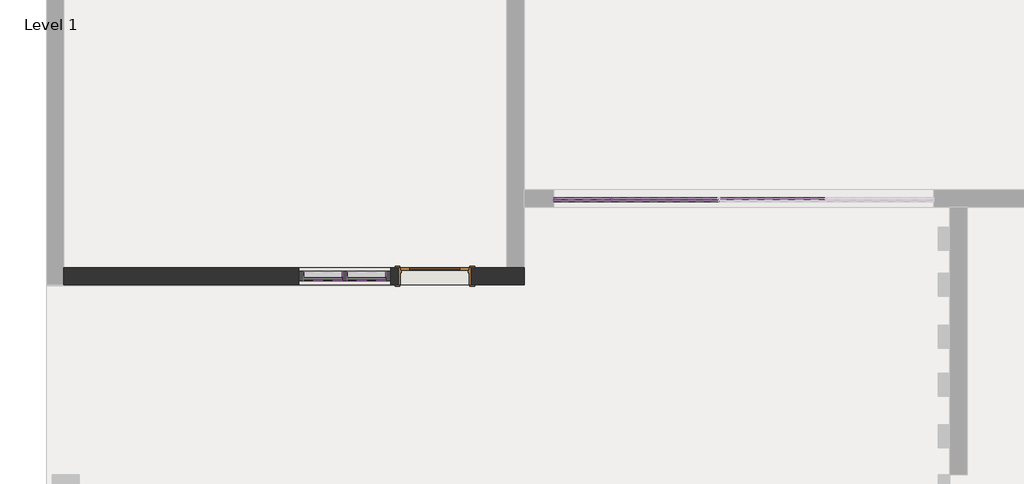
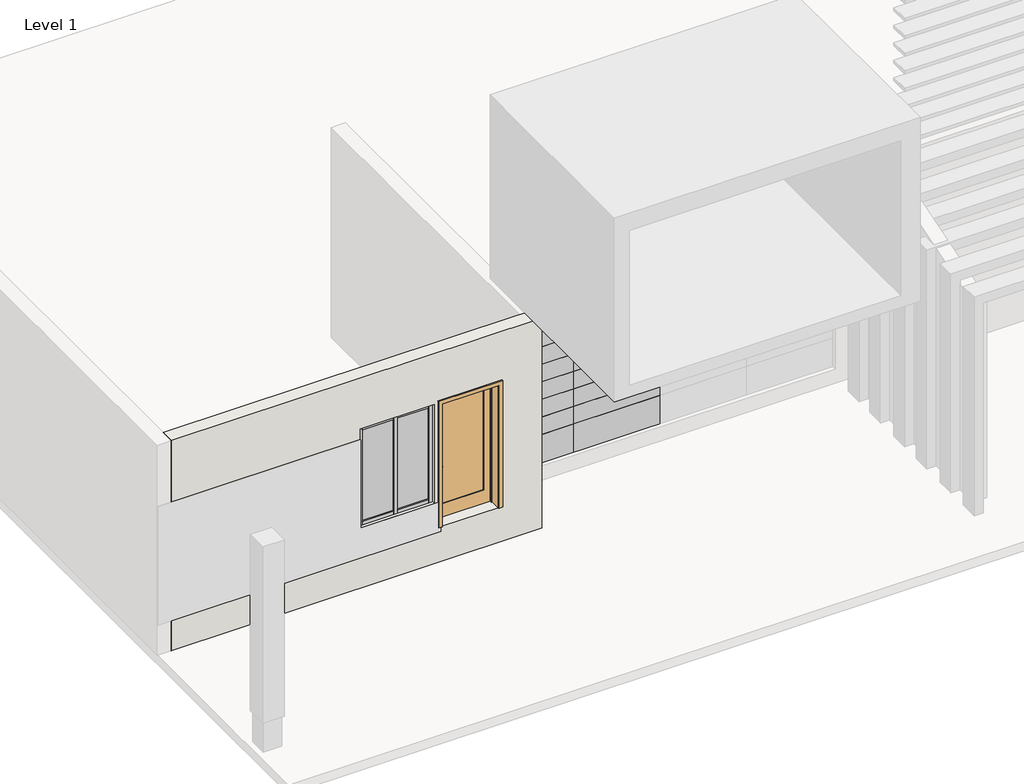
# One storey, part 1 of 2: 50 members, 18 plates, 1 door, 1 wall.
"""IFC4 building model written with IfcOpenShell, lengths in millimetres."""

from ifc_helpers import new_model, si_unit, origin, place, context, project, spatial, faceted_brep, transform, mapped, element, save
from components import door_interior_single_1_panel_wood_3_x_7_3b97b8e7, member_f362a377, member_550490f7, member_dc2600c8, member_5ac041f4, member_20a2445f, member_63f4cac5, member_d020295e, member_84e80635, member_b7a731ef, member_839e3c67, member_0b7646a3, member_58564e40, member_14ac651b, system_panel_glazed_f636780f, system_panel_glazed_497abead, system_panel_glazed_074527c7, system_panel_glazed_4c8acbbb, system_panel_glazed_d4e05dc3, system_panel_glazed_d663d970, system_panel_glazed_cac74210

model = new_model("IFC4")

# Units and contexts
model_context = context("Model", 3, world=origin())
ifc_project = project(units=[si_unit("LENGTHUNIT", "METRE", prefix="MILLI")], contexts=[model_context])

# Site, building, storey
site = spatial("IfcSite", under=ifc_project)
building = spatial("IfcBuilding", under=site)
storey = spatial("IfcBuildingStorey", under=building, Name="Level 1", Elevation=0.0)

# Door
placement = place(None, origin())
door_interior_single_1_panel_wood_3_x_7_shape = door_interior_single_1_panel_wood_3_x_7_3b97b8e7(model_context)
element("IfcDoor", 1, ObjectType="Door-Interior-Single-1_Panel-Wood : 3' x 7'", at=placement, inside=storey, context=model_context, shape_type="MappedRepresentation", body=[
    mapped(door_interior_single_1_panel_wood_3_x_7_shape, transform((-8192.4294011, -2264.4361529, 609.6), x_axis=(1.0, 0.0, 0.0), y_axis=(0.0, 1.0, 0.0), z_axis=(0.0, 0.0, 1.0))),
])

# Members
member_shape = member_f362a377(model_context)
element("IfcMember", 2, ObjectType="Rectangular Mullion : 1\" Square", at=placement, inside=storey, context=model_context, shape_type="MappedRepresentation", body=[
    mapped(member_shape, transform((-6592.2294011, -1238.9111529, 2823.4928635), x_axis=(0.0, 0.0, 1.0), y_axis=(0.0, 1.0, 0.0), z_axis=(-1.0, 0.0, 0.0))),
])
member_2_shape = member_550490f7(model_context)
element("IfcMember", 3, ObjectType="Rectangular Mullion : 1\" Square", at=placement, inside=storey, context=model_context, shape_type="MappedRepresentation", body=[
    mapped(member_2_shape, transform((-6592.2294011, -1238.9111529, 2572.3741932), x_axis=(0.0, 0.0, 1.0), y_axis=(0.0, 1.0, 0.0), z_axis=(-1.0, 0.0, 0.0))),
])
element("IfcMember", 4, ObjectType="Rectangular Mullion : 1\" Square", at=placement, inside=storey, context=model_context, shape_type="MappedRepresentation", body=[
    mapped(member_2_shape, transform((-6592.2294011, -1238.9111529, 2267.5741932), x_axis=(0.0, 0.0, 1.0), y_axis=(0.0, 1.0, 0.0), z_axis=(-1.0, 0.0, 0.0))),
])
element("IfcMember", 5, ObjectType="Rectangular Mullion : 1\" Square", at=placement, inside=storey, context=model_context, shape_type="MappedRepresentation", body=[
    mapped(member_2_shape, transform((-6592.2294011, -1238.9111529, 1962.7741932), x_axis=(0.0, 0.0, 1.0), y_axis=(0.0, 1.0, 0.0), z_axis=(-1.0, 0.0, 0.0))),
])
element("IfcMember", 6, ObjectType="Rectangular Mullion : 1\" Square", at=placement, inside=storey, context=model_context, shape_type="MappedRepresentation", body=[
    mapped(member_2_shape, transform((-6592.2294011, -1238.9111529, 1353.1741932), x_axis=(0.0, 0.0, 1.0), y_axis=(0.0, 1.0, 0.0), z_axis=(-1.0, 0.0, 0.0))),
])
element("IfcMember", 7, ObjectType="Rectangular Mullion : 1\" Square", at=placement, inside=storey, context=model_context, shape_type="MappedRepresentation", body=[
    mapped(member_2_shape, transform((-6592.2294011, -1238.9111529, 1657.9741932), x_axis=(0.0, 0.0, 1.0), y_axis=(0.0, 1.0, 0.0), z_axis=(-1.0, 0.0, 0.0))),
])
element("IfcMember", 8, ObjectType="Rectangular Mullion : 1\" Square", at=placement, inside=storey, context=model_context, shape_type="MappedRepresentation", body=[
    mapped(member_2_shape, transform((-6592.2294011, -1238.9111529, 1048.3741932), x_axis=(0.0, 0.0, 1.0), y_axis=(0.0, 1.0, 0.0), z_axis=(-1.0, 0.0, 0.0))),
])
element("IfcMember", 9, ObjectType="Rectangular Mullion : 1\" Square", at=placement, inside=storey, context=model_context, shape_type="MappedRepresentation", body=[
    mapped(member_2_shape, transform((-6592.2294011, -1238.9111529, 743.5741932), x_axis=(0.0, 0.0, 1.0), y_axis=(0.0, 1.0, 0.0), z_axis=(-1.0, 0.0, 0.0))),
])
member_3_shape = member_dc2600c8(model_context)
element("IfcMember", 10, ObjectType="Rectangular Mullion : 1\" Square", at=placement, inside=storey, context=model_context, shape_type="MappedRepresentation", body=[
    mapped(member_3_shape, transform((-5842.9294011, -1238.9111529, 2572.3741932), x_axis=(0.0, 0.0, 1.0), y_axis=(0.0, 1.0, 0.0), z_axis=(-1.0, 0.0, 0.0))),
])
element("IfcMember", 11, ObjectType="Rectangular Mullion : 1\" Square", at=placement, inside=storey, context=model_context, shape_type="MappedRepresentation", body=[
    mapped(member_3_shape, transform((-4420.5294011, -1238.9111529, 2572.3741932), x_axis=(0.0, 0.0, 1.0), y_axis=(0.0, 1.0, 0.0), z_axis=(-1.0, 0.0, 0.0))),
])
element("IfcMember", 12, ObjectType="Rectangular Mullion : 1\" Square", at=placement, inside=storey, context=model_context, shape_type="MappedRepresentation", body=[
    mapped(member_3_shape, transform((-5842.9294011, -1238.9111529, 2267.5741932), x_axis=(0.0, 0.0, 1.0), y_axis=(0.0, 1.0, 0.0), z_axis=(-1.0, 0.0, 0.0))),
])
element("IfcMember", 13, ObjectType="Rectangular Mullion : 1\" Square", at=placement, inside=storey, context=model_context, shape_type="MappedRepresentation", body=[
    mapped(member_3_shape, transform((-4420.5294011, -1238.9111529, 2267.5741932), x_axis=(0.0, 0.0, 1.0), y_axis=(0.0, 1.0, 0.0), z_axis=(-1.0, 0.0, 0.0))),
])
element("IfcMember", 14, ObjectType="Rectangular Mullion : 1\" Square", at=placement, inside=storey, context=model_context, shape_type="MappedRepresentation", body=[
    mapped(member_3_shape, transform((-5842.9294011, -1238.9111529, 1962.7741932), x_axis=(0.0, 0.0, 1.0), y_axis=(0.0, 1.0, 0.0), z_axis=(-1.0, 0.0, 0.0))),
])
element("IfcMember", 15, ObjectType="Rectangular Mullion : 1\" Square", at=placement, inside=storey, context=model_context, shape_type="MappedRepresentation", body=[
    mapped(member_3_shape, transform((-4420.5294011, -1238.9111529, 1962.7741932), x_axis=(0.0, 0.0, 1.0), y_axis=(0.0, 1.0, 0.0), z_axis=(-1.0, 0.0, 0.0))),
])
element("IfcMember", 16, ObjectType="Rectangular Mullion : 1\" Square", at=placement, inside=storey, context=model_context, shape_type="MappedRepresentation", body=[
    mapped(member_3_shape, transform((-5842.9294011, -1238.9111529, 1353.1741932), x_axis=(0.0, 0.0, 1.0), y_axis=(0.0, 1.0, 0.0), z_axis=(-1.0, 0.0, 0.0))),
])
element("IfcMember", 17, ObjectType="Rectangular Mullion : 1\" Square", at=placement, inside=storey, context=model_context, shape_type="MappedRepresentation", body=[
    mapped(member_3_shape, transform((-4420.5294011, -1238.9111529, 1353.1741932), x_axis=(0.0, 0.0, 1.0), y_axis=(0.0, 1.0, 0.0), z_axis=(-1.0, 0.0, 0.0))),
])
element("IfcMember", 18, ObjectType="Rectangular Mullion : 1\" Square", at=placement, inside=storey, context=model_context, shape_type="MappedRepresentation", body=[
    mapped(member_3_shape, transform((-5842.9294011, -1238.9111529, 1657.9741932), x_axis=(0.0, 0.0, 1.0), y_axis=(0.0, 1.0, 0.0), z_axis=(-1.0, 0.0, 0.0))),
])
element("IfcMember", 19, ObjectType="Rectangular Mullion : 1\" Square", at=placement, inside=storey, context=model_context, shape_type="MappedRepresentation", body=[
    mapped(member_3_shape, transform((-4420.5294011, -1238.9111529, 1657.9741932), x_axis=(0.0, 0.0, 1.0), y_axis=(0.0, 1.0, 0.0), z_axis=(-1.0, 0.0, 0.0))),
])
element("IfcMember", 20, ObjectType="Rectangular Mullion : 1\" Square", at=placement, inside=storey, context=model_context, shape_type="MappedRepresentation", body=[
    mapped(member_3_shape, transform((-5842.9294011, -1238.9111529, 1048.3741932), x_axis=(0.0, 0.0, 1.0), y_axis=(0.0, 1.0, 0.0), z_axis=(-1.0, 0.0, 0.0))),
])
element("IfcMember", 21, ObjectType="Rectangular Mullion : 1\" Square", at=placement, inside=storey, context=model_context, shape_type="MappedRepresentation", body=[
    mapped(member_3_shape, transform((-4420.5294011, -1238.9111529, 1048.3741932), x_axis=(0.0, 0.0, 1.0), y_axis=(0.0, 1.0, 0.0), z_axis=(-1.0, 0.0, 0.0))),
])
element("IfcMember", 22, ObjectType="Rectangular Mullion : 1\" Square", at=placement, inside=storey, context=model_context, shape_type="MappedRepresentation", body=[
    mapped(member_3_shape, transform((-5842.9294011, -1238.9111529, 743.5741932), x_axis=(0.0, 0.0, 1.0), y_axis=(0.0, 1.0, 0.0), z_axis=(-1.0, 0.0, 0.0))),
])
element("IfcMember", 23, ObjectType="Rectangular Mullion : 1\" Square", at=placement, inside=storey, context=model_context, shape_type="MappedRepresentation", body=[
    mapped(member_3_shape, transform((-4420.5294011, -1238.9111529, 743.5741932), x_axis=(0.0, 0.0, 1.0), y_axis=(0.0, 1.0, 0.0), z_axis=(-1.0, 0.0, 0.0))),
])
member_4_shape = member_5ac041f4(model_context)
element("IfcMember", 24, ObjectType="Rectangular Mullion : 1\" Square", at=placement, inside=storey, context=model_context, shape_type="MappedRepresentation", body=[
    mapped(member_4_shape, transform((-5855.6294011, -1238.9111529, 247.9343309), x_axis=(-1.0, 0.0, 0.0), y_axis=(0.0, 1.0, 0.0), z_axis=(0.0, 0.0, -1.0))),
])
element("IfcMember", 25, ObjectType="Rectangular Mullion : 1\" Square", at=placement, inside=storey, context=model_context, shape_type="MappedRepresentation", body=[
    mapped(member_4_shape, transform((-4433.2294011, -1238.9111529, 247.9343309), x_axis=(-1.0, 0.0, 0.0), y_axis=(0.0, 1.0, 0.0), z_axis=(0.0, 0.0, -1.0))),
])
element("IfcMember", 26, ObjectType="Rectangular Mullion : 1\" Square", at=placement, inside=storey, context=model_context, shape_type="MappedRepresentation", body=[
    mapped(member_shape, transform((-5868.3294011, -1238.9111529, 247.9343309), x_axis=(0.0, 0.0, -1.0), y_axis=(0.0, 1.0, 0.0), z_axis=(1.0, 0.0, 0.0))),
])
member_5_shape = member_20a2445f(model_context)
element("IfcMember", 27, ObjectType="Rectangular Mullion : 1\" Square", at=placement, inside=storey, context=model_context, shape_type="MappedRepresentation", body=[
    mapped(member_5_shape, transform((-4445.9294011, -1238.9111529, 247.9343309), x_axis=(0.0, 0.0, -1.0), y_axis=(0.0, 1.0, 0.0), z_axis=(1.0, 0.0, 0.0))),
])
element("IfcMember", 28, ObjectType="Rectangular Mullion : 1\" Square", at=placement, inside=storey, context=model_context, shape_type="MappedRepresentation", body=[
    mapped(member_5_shape, transform((-5842.9294011, -1238.9111529, 2823.4928635), x_axis=(0.0, 0.0, 1.0), y_axis=(0.0, 1.0, 0.0), z_axis=(-1.0, 0.0, 0.0))),
])
element("IfcMember", 29, ObjectType="Rectangular Mullion : 1\" Square", at=placement, inside=storey, context=model_context, shape_type="MappedRepresentation", body=[
    mapped(member_5_shape, transform((-4420.5294011, -1238.9111529, 2823.4928635), x_axis=(0.0, 0.0, 1.0), y_axis=(0.0, 1.0, 0.0), z_axis=(-1.0, 0.0, 0.0))),
])
member_6_shape = member_63f4cac5(model_context)
element("IfcMember", 30, ObjectType="Rectangular Mullion : 1\" Square", at=placement, inside=storey, context=model_context, shape_type="MappedRepresentation", body=[
    mapped(member_6_shape, transform((-5855.6294011, -1238.9111529, 2572.3741932), x_axis=(-1.0, 0.0, 0.0), y_axis=(0.0, 1.0, 0.0), z_axis=(0.0, 0.0, -1.0))),
])
member_7_shape = member_d020295e(model_context)
element("IfcMember", 31, ObjectType="Rectangular Mullion : 1\" Square", at=placement, inside=storey, context=model_context, shape_type="MappedRepresentation", body=[
    mapped(member_7_shape, transform((-5855.6294011, -1238.9111529, 2267.5741932), x_axis=(-1.0, 0.0, 0.0), y_axis=(0.0, 1.0, 0.0), z_axis=(0.0, 0.0, -1.0))),
])
element("IfcMember", 32, ObjectType="Rectangular Mullion : 1\" Square", at=placement, inside=storey, context=model_context, shape_type="MappedRepresentation", body=[
    mapped(member_7_shape, transform((-5855.6294011, -1238.9111529, 1962.7741932), x_axis=(-1.0, 0.0, 0.0), y_axis=(0.0, 1.0, 0.0), z_axis=(0.0, 0.0, -1.0))),
])
element("IfcMember", 33, ObjectType="Rectangular Mullion : 1\" Square", at=placement, inside=storey, context=model_context, shape_type="MappedRepresentation", body=[
    mapped(member_7_shape, transform((-5855.6294011, -1238.9111529, 1353.1741932), x_axis=(-1.0, 0.0, 0.0), y_axis=(0.0, 1.0, 0.0), z_axis=(0.0, 0.0, -1.0))),
])
element("IfcMember", 34, ObjectType="Rectangular Mullion : 1\" Square", at=placement, inside=storey, context=model_context, shape_type="MappedRepresentation", body=[
    mapped(member_7_shape, transform((-5855.6294011, -1238.9111529, 1657.9741932), x_axis=(-1.0, 0.0, 0.0), y_axis=(0.0, 1.0, 0.0), z_axis=(0.0, 0.0, -1.0))),
])
element("IfcMember", 35, ObjectType="Rectangular Mullion : 1\" Square", at=placement, inside=storey, context=model_context, shape_type="MappedRepresentation", body=[
    mapped(member_7_shape, transform((-5855.6294011, -1238.9111529, 1048.3741932), x_axis=(-1.0, 0.0, 0.0), y_axis=(0.0, 1.0, 0.0), z_axis=(0.0, 0.0, -1.0))),
])
element("IfcMember", 36, ObjectType="Rectangular Mullion : 1\" Square", at=placement, inside=storey, context=model_context, shape_type="MappedRepresentation", body=[
    mapped(member_7_shape, transform((-5855.6294011, -1238.9111529, 743.5741932), x_axis=(-1.0, 0.0, 0.0), y_axis=(0.0, 1.0, 0.0), z_axis=(0.0, 0.0, -1.0))),
])
member_8_shape = member_84e80635(model_context)
element("IfcMember", 37, ObjectType="Rectangular Mullion : 1\" Square", at=placement, inside=storey, context=model_context, shape_type="MappedRepresentation", body=[
    mapped(member_8_shape, transform((-6617.6294011, -1238.9111529, 247.9343309), x_axis=(-1.0, 0.0, 0.0), y_axis=(0.0, 1.0, 0.0), z_axis=(0.0, 0.0, -1.0))),
])
member_9_shape = member_b7a731ef(model_context)
element("IfcMember", 38, ObjectType="Rectangular Mullion : 1\" Square", at=placement, inside=storey, context=model_context, shape_type="MappedRepresentation", body=[
    mapped(member_9_shape, transform((-6617.6294011, -1238.9111529, 2572.3741932), x_axis=(-1.0, 0.0, 0.0), y_axis=(0.0, 1.0, 0.0), z_axis=(0.0, 0.0, -1.0))),
])
member_10_shape = member_839e3c67(model_context)
element("IfcMember", 39, ObjectType="Rectangular Mullion : 1\" Square", at=placement, inside=storey, context=model_context, shape_type="MappedRepresentation", body=[
    mapped(member_10_shape, transform((-6617.6294011, -1238.9111529, 2267.5741932), x_axis=(-1.0, 0.0, 0.0), y_axis=(0.0, 1.0, 0.0), z_axis=(0.0, 0.0, -1.0))),
])
element("IfcMember", 40, ObjectType="Rectangular Mullion : 1\" Square", at=placement, inside=storey, context=model_context, shape_type="MappedRepresentation", body=[
    mapped(member_10_shape, transform((-6617.6294011, -1238.9111529, 1962.7741932), x_axis=(-1.0, 0.0, 0.0), y_axis=(0.0, 1.0, 0.0), z_axis=(0.0, 0.0, -1.0))),
])
element("IfcMember", 41, ObjectType="Rectangular Mullion : 1\" Square", at=placement, inside=storey, context=model_context, shape_type="MappedRepresentation", body=[
    mapped(member_10_shape, transform((-6617.6294011, -1238.9111529, 1353.1741932), x_axis=(-1.0, 0.0, 0.0), y_axis=(0.0, 1.0, 0.0), z_axis=(0.0, 0.0, -1.0))),
])
element("IfcMember", 42, ObjectType="Rectangular Mullion : 1\" Square", at=placement, inside=storey, context=model_context, shape_type="MappedRepresentation", body=[
    mapped(member_10_shape, transform((-6617.6294011, -1238.9111529, 1657.9741932), x_axis=(-1.0, 0.0, 0.0), y_axis=(0.0, 1.0, 0.0), z_axis=(0.0, 0.0, -1.0))),
])
element("IfcMember", 43, ObjectType="Rectangular Mullion : 1\" Square", at=placement, inside=storey, context=model_context, shape_type="MappedRepresentation", body=[
    mapped(member_10_shape, transform((-6617.6294011, -1238.9111529, 1048.3741932), x_axis=(-1.0, 0.0, 0.0), y_axis=(0.0, 1.0, 0.0), z_axis=(0.0, 0.0, -1.0))),
])
element("IfcMember", 44, ObjectType="Rectangular Mullion : 1\" Square", at=placement, inside=storey, context=model_context, shape_type="MappedRepresentation", body=[
    mapped(member_10_shape, transform((-6617.6294011, -1238.9111529, 743.5741932), x_axis=(-1.0, 0.0, 0.0), y_axis=(0.0, 1.0, 0.0), z_axis=(0.0, 0.0, -1.0))),
])
member_11_shape = member_0b7646a3(model_context)
element("IfcMember", 45, ObjectType="Rectangular Mullion : 2.5\" x 5\" rectangular 2", at=placement, inside=storey, context=model_context, shape_type="MappedRepresentation", body=[
    mapped(member_11_shape, transform((-9932.3294011, -2267.6111529, 2768.6), x_axis=(0.0, 0.0, 1.0), y_axis=(0.0, 1.0, 0.0), z_axis=(-1.0, 0.0, 0.0))),
])
element("IfcMember", 46, ObjectType="Rectangular Mullion : 2.5\" x 5\" rectangular 2", at=placement, inside=storey, context=model_context, shape_type="MappedRepresentation", body=[
    mapped(member_11_shape, transform((-9354.4794011, -2267.6111529, 2768.6), x_axis=(0.0, 0.0, 1.0), y_axis=(0.0, 1.0, 0.0), z_axis=(-1.0, 0.0, 0.0))),
])
element("IfcMember", 47, ObjectType="Rectangular Mullion : 2.5\" x 5\" rectangular 2", at=placement, inside=storey, context=model_context, shape_type="MappedRepresentation", body=[
    mapped(member_11_shape, transform((-8840.1294011, -2267.6111529, 1047.6775384), x_axis=(0.0, 0.0, -1.0), y_axis=(0.0, 1.0, 0.0), z_axis=(1.0, 0.0, 0.0))),
])
element("IfcMember", 48, ObjectType="Rectangular Mullion : 2.5\" x 5\" rectangular 2", at=placement, inside=storey, context=model_context, shape_type="MappedRepresentation", body=[
    mapped(member_11_shape, transform((-9417.9794011, -2267.6111529, 1047.6775384), x_axis=(0.0, 0.0, -1.0), y_axis=(0.0, 1.0, 0.0), z_axis=(1.0, 0.0, 0.0))),
])
member_12_shape = member_58564e40(model_context)
element("IfcMember", 49, ObjectType="Rectangular Mullion : 2.5\" x 5\" rectangular 2", at=placement, inside=storey, context=model_context, shape_type="MappedRepresentation", body=[
    mapped(member_12_shape, transform((-9386.2294011, -2267.6111529, 1047.6775384), x_axis=(-1.0, 0.0, 0.0), y_axis=(0.0, 1.0, 0.0), z_axis=(0.0, 0.0, -1.0))),
])
member_13_shape = member_14ac651b(model_context)
element("IfcMember", 50, ObjectType="Rectangular Mullion : 2.5\" x 5\" rectangular 2", at=placement, inside=storey, context=model_context, shape_type="MappedRepresentation", body=[
    mapped(member_13_shape, transform((-8776.6294011, -2267.6111529, 2768.6), x_axis=(1.0, 0.0, 0.0), y_axis=(0.0, 1.0, 0.0), z_axis=(0.0, 0.0, 1.0))),
])
element("IfcMember", 51, ObjectType="Rectangular Mullion : 2.5\" x 5\" rectangular 2", at=placement, inside=storey, context=model_context, shape_type="MappedRepresentation", body=[
    mapped(member_13_shape, transform((-9995.8294011, -2267.6111529, 1047.6775384), x_axis=(-1.0, 0.0, 0.0), y_axis=(0.0, 1.0, 0.0), z_axis=(0.0, 0.0, -1.0))),
])

# Plates
system_panel_glazed_shape = system_panel_glazed_f636780f(model_context)
element("IfcPlate", 52, ObjectType="System Panel : Glazed", at=placement, inside=storey, context=model_context, shape_type="MappedRepresentation", body=[
    mapped(system_panel_glazed_shape, transform((-9097.3044011, -2267.6111529, 1111.1775384), x_axis=(-1.0, 0.0, 0.0), y_axis=(0.0, -1.0, 0.0), z_axis=(0.0, 0.0, 1.0))),
])
element("IfcPlate", 53, ObjectType="System Panel : Glazed", at=placement, inside=storey, context=model_context, shape_type="MappedRepresentation", body=[
    mapped(system_panel_glazed_shape, transform((-9675.1544011, -2267.6111529, 1111.1775384), x_axis=(-1.0, 0.0, 0.0), y_axis=(0.0, -1.0, 0.0), z_axis=(0.0, 0.0, 1.0))),
])
system_panel_glazed_2_shape = system_panel_glazed_497abead(model_context)
element("IfcPlate", 54, ObjectType="System Panel : Glazed", at=placement, inside=storey, context=model_context, shape_type="MappedRepresentation", body=[
    mapped(system_panel_glazed_2_shape, transform((-6236.6294011, -1238.9111529, 247.9343309), x_axis=(-1.0, 0.0, 0.0), y_axis=(0.0, -1.0, 0.0), z_axis=(0.0, 0.0, 1.0))),
])
system_panel_glazed_3_shape = system_panel_glazed_074527c7(model_context)
element("IfcPlate", 55, ObjectType="System Panel : Glazed", at=placement, inside=storey, context=model_context, shape_type="MappedRepresentation", body=[
    mapped(system_panel_glazed_3_shape, transform((-6236.6294011, -1238.9111529, 743.5741932), x_axis=(-1.0, 0.0, 0.0), y_axis=(0.0, -1.0, 0.0), z_axis=(0.0, 0.0, 1.0))),
])
element("IfcPlate", 56, ObjectType="System Panel : Glazed", at=placement, inside=storey, context=model_context, shape_type="MappedRepresentation", body=[
    mapped(system_panel_glazed_3_shape, transform((-6236.6294011, -1238.9111529, 1048.3741932), x_axis=(-1.0, 0.0, 0.0), y_axis=(0.0, -1.0, 0.0), z_axis=(0.0, 0.0, 1.0))),
])
element("IfcPlate", 57, ObjectType="System Panel : Glazed", at=placement, inside=storey, context=model_context, shape_type="MappedRepresentation", body=[
    mapped(system_panel_glazed_3_shape, transform((-6236.6294011, -1238.9111529, 1353.1741932), x_axis=(-1.0, 0.0, 0.0), y_axis=(0.0, -1.0, 0.0), z_axis=(0.0, 0.0, 1.0))),
])
element("IfcPlate", 58, ObjectType="System Panel : Glazed", at=placement, inside=storey, context=model_context, shape_type="MappedRepresentation", body=[
    mapped(system_panel_glazed_3_shape, transform((-6236.6294011, -1238.9111529, 1657.9741932), x_axis=(-1.0, 0.0, 0.0), y_axis=(0.0, -1.0, 0.0), z_axis=(0.0, 0.0, 1.0))),
])
element("IfcPlate", 59, ObjectType="System Panel : Glazed", at=placement, inside=storey, context=model_context, shape_type="MappedRepresentation", body=[
    mapped(system_panel_glazed_3_shape, transform((-6236.6294011, -1238.9111529, 1962.7741932), x_axis=(-1.0, 0.0, 0.0), y_axis=(0.0, -1.0, 0.0), z_axis=(0.0, 0.0, 1.0))),
])
element("IfcPlate", 60, ObjectType="System Panel : Glazed", at=placement, inside=storey, context=model_context, shape_type="MappedRepresentation", body=[
    mapped(system_panel_glazed_3_shape, transform((-6236.6294011, -1238.9111529, 2267.5741932), x_axis=(-1.0, 0.0, 0.0), y_axis=(0.0, -1.0, 0.0), z_axis=(0.0, 0.0, 1.0))),
])
system_panel_glazed_4_shape = system_panel_glazed_4c8acbbb(model_context)
element("IfcPlate", 61, ObjectType="System Panel : Glazed", at=placement, inside=storey, context=model_context, shape_type="MappedRepresentation", body=[
    mapped(system_panel_glazed_4_shape, transform((-6236.6294011, -1238.9111529, 2572.3741932), x_axis=(-1.0, 0.0, 0.0), y_axis=(0.0, -1.0, 0.0), z_axis=(0.0, 0.0, 1.0))),
])
system_panel_glazed_5_shape = system_panel_glazed_d4e05dc3(model_context)
element("IfcPlate", 62, ObjectType="System Panel : Glazed", at=placement, inside=storey, context=model_context, shape_type="MappedRepresentation", body=[
    mapped(system_panel_glazed_5_shape, transform((-5144.4294011, -1238.9111529, 247.9343309), x_axis=(-1.0, 0.0, 0.0), y_axis=(0.0, -1.0, 0.0), z_axis=(0.0, 0.0, 1.0))),
])
system_panel_glazed_6_shape = system_panel_glazed_d663d970(model_context)
element("IfcPlate", 63, ObjectType="System Panel : Glazed", at=placement, inside=storey, context=model_context, shape_type="MappedRepresentation", body=[
    mapped(system_panel_glazed_6_shape, transform((-5144.4294011, -1238.9111529, 743.5741932), x_axis=(-1.0, 0.0, 0.0), y_axis=(0.0, -1.0, 0.0), z_axis=(0.0, 0.0, 1.0))),
])
element("IfcPlate", 64, ObjectType="System Panel : Glazed", at=placement, inside=storey, context=model_context, shape_type="MappedRepresentation", body=[
    mapped(system_panel_glazed_6_shape, transform((-5144.4294011, -1238.9111529, 1048.3741932), x_axis=(-1.0, 0.0, 0.0), y_axis=(0.0, -1.0, 0.0), z_axis=(0.0, 0.0, 1.0))),
])
element("IfcPlate", 65, ObjectType="System Panel : Glazed", at=placement, inside=storey, context=model_context, shape_type="MappedRepresentation", body=[
    mapped(system_panel_glazed_6_shape, transform((-5144.4294011, -1238.9111529, 1353.1741932), x_axis=(-1.0, 0.0, 0.0), y_axis=(0.0, -1.0, 0.0), z_axis=(0.0, 0.0, 1.0))),
])
element("IfcPlate", 66, ObjectType="System Panel : Glazed", at=placement, inside=storey, context=model_context, shape_type="MappedRepresentation", body=[
    mapped(system_panel_glazed_6_shape, transform((-5144.4294011, -1238.9111529, 1657.9741932), x_axis=(-1.0, 0.0, 0.0), y_axis=(0.0, -1.0, 0.0), z_axis=(0.0, 0.0, 1.0))),
])
element("IfcPlate", 67, ObjectType="System Panel : Glazed", at=placement, inside=storey, context=model_context, shape_type="MappedRepresentation", body=[
    mapped(system_panel_glazed_6_shape, transform((-5144.4294011, -1238.9111529, 1962.7741932), x_axis=(-1.0, 0.0, 0.0), y_axis=(0.0, -1.0, 0.0), z_axis=(0.0, 0.0, 1.0))),
])
element("IfcPlate", 68, ObjectType="System Panel : Glazed", at=placement, inside=storey, context=model_context, shape_type="MappedRepresentation", body=[
    mapped(system_panel_glazed_6_shape, transform((-5144.4294011, -1238.9111529, 2267.5741932), x_axis=(-1.0, 0.0, 0.0), y_axis=(0.0, -1.0, 0.0), z_axis=(0.0, 0.0, 1.0))),
])
system_panel_glazed_7_shape = system_panel_glazed_cac74210(model_context)
element("IfcPlate", 69, ObjectType="System Panel : Glazed", at=placement, inside=storey, context=model_context, shape_type="MappedRepresentation", body=[
    mapped(system_panel_glazed_7_shape, transform((-5144.4294011, -1238.9111529, 2572.3741932), x_axis=(-1.0, 0.0, 0.0), y_axis=(0.0, -1.0, 0.0), z_axis=(0.0, 0.0, 1.0))),
])

# Wall
element("IfcWall", 70, ObjectType="9\" wall", at=placement, inside=storey, context=model_context, shape_type="Brep", body=[
    faceted_brep([(-13107.3294011, -2381.9111529, 0.0), (-7011.3294011, -2381.9111529, 0.0), (-7011.3294011, -2381.9111529, 3657.6), (-13107.3294011, -2381.9111529, 3657.6), (-7709.8294011, -2381.9111529, 2768.6), (-7709.8294011, -2381.9111529, 609.6), (-8675.0294011, -2381.9111529, 609.6), (-8675.0294011, -2381.9111529, 2768.6), (-8776.6294011, -2381.9111529, 2768.6), (-8776.6294011, -2381.9111529, 1047.6775384), (-9995.8294011, -2381.9111529, 1047.6775384), (-9995.8294011, -2381.9111529, 2768.6), (-7011.3294011, -2153.3111529, 0.0), (-7239.9294011, -2153.3111529, 0.0), (-13107.3294011, -2153.3111529, 0.0), (-13107.3294011, -2153.3111529, 3657.6), (-7239.9294011, -2153.3111529, 3657.6), (-7011.3294011, -2153.3111529, 3657.6), (-7709.8294011, -2153.3111529, 609.6), (-7709.8294011, -2153.3111529, 2768.6), (-8675.0294011, -2153.3111529, 2768.6), (-8675.0294011, -2153.3111529, 609.6), (-8776.6294011, -2153.3111529, 1047.6775384), (-8776.6294011, -2153.3111529, 2768.6), (-9995.8294011, -2153.3111529, 2768.6), (-9995.8294011, -2153.3111529, 1047.6775384)], [[[0, 1, 2, 3], [4, 5, 6, 7], [8, 9, 10, 11]], [[12, 13, 14, 15, 16, 17], [18, 19, 20, 21], [22, 23, 24, 25]], [[1, 0, 14, 13, 12]], [[3, 2, 17, 16, 15]], [[0, 3, 15, 14]], [[2, 1, 12, 17]], [[18, 5, 4, 19]], [[19, 4, 7, 20]], [[6, 21, 20, 7]], [[5, 18, 21, 6]], [[22, 9, 8, 23]], [[23, 8, 11, 24]], [[24, 11, 10, 25]], [[9, 22, 25, 10]]]),
])

save(model, "model.ifc")

# Revit data of these elements
# Type "Door-Interior-Single-1_Panel-Wood : 3' x 7'"
#   Type Mark = "9"
#   Assembly Code = "C1020300"
#   Analytic Construction = "Wooden"
#   Top Rail = 0' - 4 11/16"
#   Thickness = 0' - 1 3/8"
#   Thermal Resistance (R) = 2.5876 (h·ft²·°F)/BTU
#   Swing Angle [instance default] = 90.00°
#   Stiles = 0' - 4 3/4"
#   Rough Width = 3' - 2"
#   Rough Height = 7' - 1"
#   Height = 7' - 0"
#   Width = 3' - 0"
#   Heat Transfer Coefficient (U) = 0.3865 BTU/(h·ft²·°F)
#   Bottom Rail = 0' - 9 1/8"
#   Trim Material = Cherry
#   Panel Material = Cherry
#   Frame Material = Cherry
#   Door Handle Material = Aluminum
#   Visual Light Transmittance = 0
#   Solar Heat Gain Coefficient = 0
#   Wall Closure = (empty or 0)
#   Function = (empty or 0)
# Type "Rectangular Mullion : 1\" Square"
#   built-in parameter 1007304 = 0.0833333 (stored number, unit not read)
#   built-in parameter 1007301 = 0.0416667 (stored number, unit not read)
#   built-in parameter 1007300 = 0.0416667 (stored number, unit not read)
# Type "Rectangular Mullion : 2.5\" x 5\" rectangular 2"
#   built-in parameter 1007304 = 0.416667 (stored number, unit not read)
#   built-in parameter 1007301 = 0.104167 (stored number, unit not read)
#   built-in parameter 1007300 = 0.104167 (stored number, unit not read)
# Type "System Panel : Glazed"
#   Construction Type Id = "GSP4R"
#   Analytic Construction = "1/8 in Pilkington single glazing"
#   Visual Light Transmittance = 0.9
#   Solar Heat Gain Coefficient = 0.86
#   Heat Transfer Coefficient (U) = 1.18115 BTU/(h·ft²·°F)
#   Define Thermal Properties by = 1
# Type "9\" wall"
#   Assembly Code = "B2010"
#   Layers, outside or top first: 0' - 9" "Gypsum Wall Board" (function 1)
# Element 1 (IfcDoor, "Door-Interior-Single-1_Panel-Wood : 3' x 7'")
#   Swing Angle = 90.00°
#   Phase Created = New Construction
#   Materials on its faces: "Cherry", "Aluminum"
# Elements 2, 3, 4, 5, 6, 7, 8, 9, 10, 11, 12, 13, 14, 15, 16, 17, 18, 19, 20, 21, 22, 23, 24, 25, 26, 27, 28, 29, 30, 31, 32, 33, 34, 35, 36, 37, 38, 39, 40, 41, 42, 43, 44 (IfcMember, "Rectangular Mullion : 1\" Square")
#   Phase Created = New Construction
# Elements 45, 46, 47, 48, 49, 50, 51 (IfcMember, "Rectangular Mullion : 2.5\" x 5\" rectangular 2")
#   Phase Created = New Construction
# Elements 52, 53, 54, 55, 56, 57, 58, 59, 60, 61, 62, 63, 64, 65, 66, 67, 68, 69 (IfcPlate, "System Panel : Glazed")
#   Phase Created = New Construction
#   Materials on its faces: "Glass"
# Element 70 (IfcWall, "9\" wall")
#   Top Offset = 0' - 0"
#   Base Offset = 0' - 0"
#   wall height = 12' - 0"
#   Phase Created = New Construction
#   Base Constraint = Level 1
#   Top Constraint = Level 2
#   Materials on its faces: "Gypsum Wall Board"
# Materials
#   "Cherry": class "Wood", colour RGB 226 177 128, transparency 0, Description = "Prunus Serotina", Cost = 0
#   "Aluminum": class "Metal", colour RGB 247 247 247, transparency 0, Description = "Aluminum 6061", Cost = 0
#   "Gypsum Wall Board": class "Generic", colour RGB 127 127 127, transparency 0, Description = "Gypsum Wall Board", Cost = 0
#   "Glass": class "Glass", colour RGB 0 128 192, transparency 0.75, Description = "Soda Lime Glass", Cost = 0
